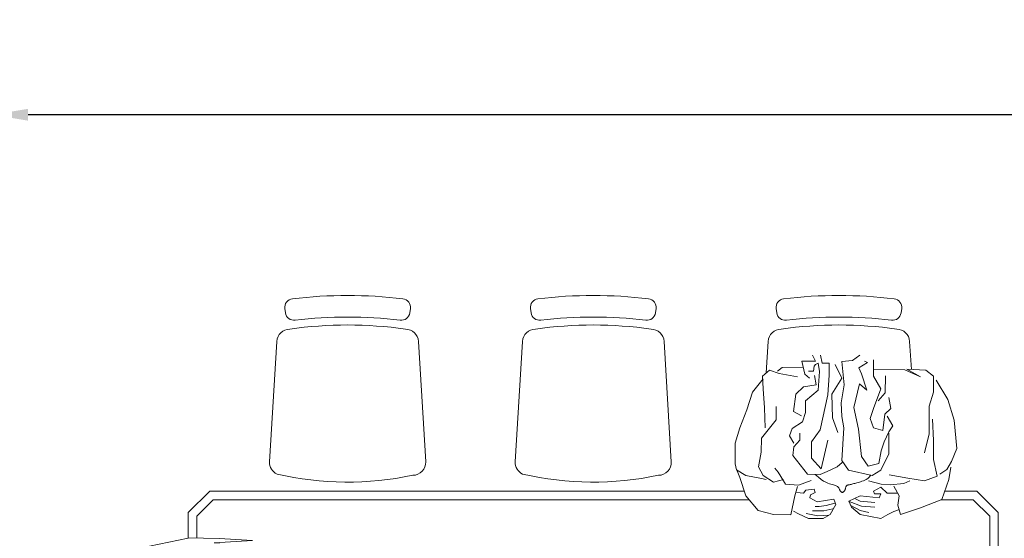
# Model space of a CAD drawing. Units: inches. Extents: x 1913 to 5309, y 1003 to 1733.
# Tile 18 of 23: x 4205 to 4275, y 1452 to 1489. Entities that reach past the tile are written whole.
import ezdxf

# ---------------------------------------------------------------- set-up
doc = ezdxf.new("R2010")
doc.units = ezdxf.units.IN
doc.layers.add('A-ANNO-DIMS', color=2, linetype='Continuous', lineweight=18)
doc.layers.add('A-FURN', color=8, linetype='Continuous', lineweight=18)
doc.styles.get("Standard").update_dxf_attribs({"font": 'arial.ttf'})
doc.dimstyles.new('ISO-25', dxfattribs={"dimtxt": 8, "dimasz": 2.5, "dimexe": 1.25, "dimexo": 0.625, "dimtad": 1, "dimdec": 1, "dimlunit": 3, "dimtxsty": 'Standard', "dimcen": 2.5, "dimclrd": 256, "dimclrt": 1, "dimadec": 0, "dimazin": 0, "dimtfac": 1, "dimtdec": 1, "dimtmove": 0, "dimatfit": 3, "dimfxl": 1, "dimarcsym": 0})

# ---------------------------------------------------------------- blocks, each defined once
blk = doc.blocks.new('A$C421907B3')
for p, q in [((1.2447, 2.3435), (1.2266, 2.4332)), ((1.4171, 1.0745), (1.4031, 1.0709)), ((1.4656, 1.0745), (1.4171, 1.0745)), ((1.5014, 1.0634), (1.4656, 1.0745)), ((1.3433, 1.0498), (1.3858, 1.0635)), ((1.3858, 1.0635), (1.4011, 1.0699)), ((1.4031, 1.0709), (1.3905, 1.0498)), ((1.5426, 1.0469), (1.5014, 1.0634)), ((1.3094, 1.0205), (1.3433, 1.0498)), ((1.3905, 1.0498), (1.3831, 1.0131)), ((1.5838, 1.034), (1.5426, 1.0469)), ((1.615, 1.0092), (1.5838, 1.034)), ((1.3001, 0.9856), (1.3094, 1.0205)), ((1.3751, 0.9856), (1.3904, 1.0094)), ((1.3831, 1.0131), (1.3811, 1.0021)), ((1.3904, 1.0094), (1.4104, 1.0204)), ((1.4104, 1.0204), (1.4443, 1.0139)), ((1.4443, 1.0139), (1.4768, 1.013)), ((1.4768, 1.013), (1.5193, 0.979)), ((1.5014, 1.0047), (1.5472, 1.0065)), ((1.5472, 1.0065), (1.5918, 1.0092)), ((1.5918, 1.0092), (1.621, 1.011)), ((1.621, 1.011), (1.6349, 0.9945)), ((1.2987, 0.9453), (1.3001, 0.9856)), ((1.3811, 0.9617), (1.3751, 0.9856)), ((1.6349, 0.9945), (1.627, 0.9725)), ((1.3705, 0.9571), (1.3877, 0.9681)), ((1.3877, 0.9681), (1.3984, 0.9745)), ((1.3984, 0.9745), (1.4077, 0.9819)), ((1.5193, 0.979), (1.5505, 0.979)), ((1.627, 0.9725), (1.6196, 0.9294)), ((1.6409, 0.9652), (1.6329, 0.9762)), ((1.6421, 0.9163), (1.6409, 0.9652)), ((1.3432, 0.9361), (1.2987, 0.9453)), ((1.3013, 0.9269), (1.3073, 0.9388)), ((1.3678, 0.9269), (1.3705, 0.9571)), ((1.3937, 0.9067), (1.4369, 0.9406)), ((1.4369, 0.9406), (1.4568, 0.9378)), ((1.4568, 0.9378), (1.4721, 0.924)), ((1.4655, 0.9378), (1.4827, 0.9479)), ((1.4827, 0.9479), (1.4994, 0.9423)), ((1.4994, 0.9423), (1.5146, 0.9176)), ((1.5286, 0.9203), (1.5392, 0.9386)), ((1.5392, 0.9386), (1.5791, 0.9331)), ((1.2907, 0.904), (1.3013, 0.9269)), ((1.3645, 0.9296), (1.3432, 0.9361)), ((1.3505, 0.9315), (1.3492, 0.9159)), ((1.3492, 0.9159), (1.3565, 0.9104)), ((1.3784, 0.8975), (1.3678, 0.9269)), ((1.4721, 0.924), (1.4887, 0.924)), ((1.5146, 0.9176), (1.5365, 0.9111)), ((1.5791, 0.9331), (1.5963, 0.9157)), ((1.5963, 0.9157), (1.601, 0.8863)), ((1.6256, 0.9129), (1.6561, 0.9193)), ((1.6561, 0.9193), (1.6561, 0.8881)), ((1.2906, 0.87), (1.2907, 0.904)), ((1.2965, 0.8821), (1.3022, 0.9091)), ((1.3079, 0.8681), (1.3079, 0.8945)), ((1.3385, 0.9012), (1.3292, 0.8838)), ((1.3458, 0.8994), (1.3385, 0.9012)), ((1.3505, 0.8883), (1.3458, 0.8994)), ((1.3565, 0.9104), (1.3584, 0.8911)), ((1.3923, 0.8773), (1.3937, 0.9067)), ((1.4056, 0.8745), (1.4302, 0.8974)), ((1.4302, 0.8974), (1.4687, 0.8974)), ((1.4687, 0.8974), (1.4966, 0.8772)), ((1.5365, 0.9111), (1.5638, 0.9111)), ((1.5638, 0.9111), (1.5883, 0.8817)), ((1.6163, 0.9019), (1.6256, 0.9129)), ((1.6329, 0.8927), (1.6329, 0.9037)), ((1.6442, 0.8908), (1.6329, 0.8927)), ((1.6561, 0.8881), (1.6701, 0.8945)), ((1.2999, 0.8535), (1.2906, 0.87)), ((1.2985, 0.8577), (1.2965, 0.8821)), ((1.3183, 0.8795), (1.3183, 0.8888)), ((1.3209, 0.8634), (1.3183, 0.8795)), ((1.3292, 0.8838), (1.3351, 0.8452)), ((1.3584, 0.8911), (1.3505, 0.8883)), ((1.3746, 0.864), (1.3774, 0.869)), ((1.3774, 0.869), (1.3812, 0.8747)), ((1.3812, 0.8747), (1.3861, 0.8811)), ((1.3861, 0.8811), (1.3923, 0.8883)), ((1.3996, 0.8608), (1.3923, 0.8773)), ((1.472, 0.8589), (1.4056, 0.8745)), ((1.4966, 0.8772), (1.5777, 0.8588)), ((1.5883, 0.8817), (1.6315, 0.8789)), ((1.601, 0.8863), (1.6222, 0.8899)), ((1.6315, 0.8789), (1.6515, 0.8817)), ((1.6481, 0.8881), (1.6442, 0.8908)), ((1.6515, 0.8817), (1.6481, 0.8881)), ((1.6514, 0.8725), (1.6701, 0.8761)), ((1.6514, 0.856), (1.6514, 0.8725)), ((1.3232, 0.8407), (1.2999, 0.8535)), ((1.3126, 0.8473), (1.3079, 0.8681)), ((1.3261, 0.8427), (1.3209, 0.8634)), ((1.368, 0.8438), (1.3687, 0.8462)), ((1.3687, 0.8462), (1.3694, 0.849)), ((1.3694, 0.849), (1.3702, 0.852)), ((1.3702, 0.852), (1.3712, 0.8555)), ((1.3712, 0.8555), (1.3726, 0.8595)), ((1.3726, 0.8595), (1.3746, 0.864)), ((1.4102, 0.8378), (1.3996, 0.8608)), ((1.49, 0.8359), (1.5239, 0.8487)), ((1.5239, 0.8487), (1.579, 0.8496)), ((1.5777, 0.8588), (1.6235, 0.856)), ((1.579, 0.8496), (1.6162, 0.8266)), ((1.6235, 0.856), (1.6514, 0.856)), ((1.3351, 0.8452), (1.3232, 0.8407)), ((1.3512, 0.826), (1.3514, 0.8269)), ((1.3512, 0.8251), (1.3512, 0.826)), ((1.3514, 0.8243), (1.3512, 0.8251)), ((1.3514, 0.8269), (1.3518, 0.8277)), ((1.3518, 0.8234), (1.3514, 0.8243)), ((1.3518, 0.8277), (1.3524, 0.8285)), ((1.3524, 0.8226), (1.3518, 0.8234)), ((1.3524, 0.8285), (1.353, 0.8292)), ((1.353, 0.8292), (1.3538, 0.8299)), ((1.3538, 0.8299), (1.3547, 0.8305)), ((1.3547, 0.8305), (1.3557, 0.8311)), ((1.3557, 0.8311), (1.3568, 0.8316)), ((1.3568, 0.8316), (1.3579, 0.832)), ((1.3579, 0.832), (1.3591, 0.8325)), ((1.3591, 0.8325), (1.3602, 0.833)), ((1.3602, 0.833), (1.3613, 0.8335)), ((1.3613, 0.8335), (1.3624, 0.8342)), ((1.3624, 0.8342), (1.3634, 0.835)), ((1.3634, 0.835), (1.3643, 0.8359)), ((1.3643, 0.8359), (1.3651, 0.837)), ((1.3651, 0.837), (1.3659, 0.8384)), ((1.3659, 0.8384), (1.3666, 0.8399)), ((1.3666, 0.8399), (1.3673, 0.8417)), ((1.3673, 0.8417), (1.368, 0.8438)), ((1.4029, 0.8112), (1.4255, 0.8268)), ((1.4208, 0.8259), (1.4102, 0.8378)), ((1.4255, 0.8268), (1.5012, 0.8222)), ((1.5012, 0.8222), (1.5272, 0.8267)), ((1.5272, 0.8267), (1.5591, 0.8285)), ((1.5591, 0.8285), (1.6009, 0.8212)), ((1.6009, 0.8212), (1.6547, 0.8266)), ((1.6162, 0.8266), (1.6481, 0.8422)), ((1.6547, 0.8266), (1.6574, 0.8018)), ((1.2999, 0.7838), (1.3165, 0.804)), ((1.3089, 0.784), (1.3203, 0.8058)), ((1.3165, 0.804), (1.3305, 0.8104)), ((1.3193, 0.7809), (1.3297, 0.8099)), ((1.3305, 0.8104), (1.3431, 0.7838)), ((1.3531, 0.8218), (1.3524, 0.8226)), ((1.354, 0.8211), (1.3531, 0.8218)), ((1.355, 0.8204), (1.354, 0.8211)), ((1.3561, 0.8198), (1.355, 0.8204)), ((1.3572, 0.8192), (1.3561, 0.8198)), ((1.3584, 0.8188), (1.3572, 0.8192)), ((1.3595, 0.8184), (1.3584, 0.8188)), ((1.3607, 0.8181), (1.3595, 0.8184)), ((1.3618, 0.8179), (1.3607, 0.8181)), ((1.3629, 0.8176), (1.3618, 0.8179)), ((1.3639, 0.8173), (1.3629, 0.8176)), ((1.3648, 0.8169), (1.3639, 0.8173)), ((1.3656, 0.8165), (1.3648, 0.8169)), ((1.3664, 0.8159), (1.3656, 0.8165)), ((1.367, 0.8151), (1.3664, 0.8159)), ((1.3675, 0.8141), (1.367, 0.8151)), ((1.3679, 0.813), (1.3675, 0.8141)), ((1.3683, 0.8118), (1.3679, 0.813)), ((1.3686, 0.8104), (1.3683, 0.8118)), ((1.369, 0.8088), (1.3686, 0.8104)), ((1.3694, 0.8071), (1.369, 0.8088)), ((1.3698, 0.8053), (1.3694, 0.8071)), ((1.3703, 0.8033), (1.3698, 0.8053)), ((1.3708, 0.8013), (1.3703, 0.8033)), ((1.3714, 0.799), (1.3708, 0.8013)), ((1.3902, 0.7562), (1.4029, 0.8112)), ((1.6574, 0.8018), (1.67, 0.7853)), ((1.2905, 0.7361), (1.2999, 0.7838)), ((1.3047, 0.7638), (1.3089, 0.784)), ((1.3166, 0.7498), (1.3193, 0.7809)), ((1.3275, 0.7498), (1.3307, 0.784)), ((1.3307, 0.784), (1.3359, 0.7949)), ((1.3431, 0.7838), (1.3384, 0.7397)), ((1.3721, 0.7967), (1.3714, 0.799)), ((1.3728, 0.7942), (1.3721, 0.7967)), ((1.3736, 0.7916), (1.3728, 0.7942)), ((1.3743, 0.7889), (1.3736, 0.7916)), ((1.3751, 0.786), (1.3743, 0.7889)), ((1.376, 0.783), (1.3751, 0.786)), ((1.3769, 0.7799), (1.376, 0.783)), ((1.378, 0.7767), (1.3769, 0.7799)), ((1.4122, 0.7654), (1.4348, 0.7809)), ((1.4348, 0.7809), (1.4979, 0.7882)), ((1.4979, 0.7882), (1.5484, 0.7992)), ((1.5484, 0.7992), (1.6035, 0.7854)), ((1.6035, 0.7854), (1.5882, 0.7689)), ((1.5882, 0.7689), (1.6268, 0.7808)), ((1.6268, 0.7808), (1.6407, 0.7872)), ((1.6407, 0.7872), (1.6527, 0.767)), ((1.3703, 0.7351), (1.3783, 0.7645)), ((1.3795, 0.7735), (1.378, 0.7767)), ((1.3813, 0.7701), (1.3795, 0.7735)), ((1.3837, 0.7667), (1.3813, 0.7701)), ((1.3866, 0.7633), (1.3837, 0.7667)), ((1.3902, 0.7599), (1.3866, 0.7633)), ((1.4028, 0.736), (1.3902, 0.7562)), ((1.4181, 0.7406), (1.4122, 0.7654)), ((1.5012, 0.7534), (1.5224, 0.7607)), ((1.5224, 0.7607), (1.5457, 0.7533)), ((1.6527, 0.767), (1.656, 0.7743)), ((1.2998, 0.7196), (1.2905, 0.7361)), ((1.3384, 0.7397), (1.3477, 0.7361)), ((1.3477, 0.7507), (1.3537, 0.7535)), ((1.3477, 0.7361), (1.3477, 0.7507)), ((1.363, 0.736), (1.349, 0.7214)), ((1.3537, 0.7535), (1.363, 0.736)), ((1.3689, 0.7149), (1.3703, 0.7351)), ((1.4407, 0.7176), (1.4028, 0.736)), ((1.4473, 0.7351), (1.4181, 0.7406)), ((1.4686, 0.7286), (1.4473, 0.7351)), ((1.4945, 0.7313), (1.5012, 0.7534)), ((1.5331, 0.7267), (1.4945, 0.7313)), ((1.5457, 0.7533), (1.5915, 0.7358)), ((1.5822, 0.7258), (1.5636, 0.7423)), ((1.5915, 0.7358), (1.6208, 0.7532)), ((1.6208, 0.7532), (1.6593, 0.7532)), ((1.6361, 0.7532), (1.636, 0.6808)), ((1.3071, 0.7058), (1.2998, 0.7196)), ((1.349, 0.7214), (1.349, 0.6984)), ((1.3716, 0.6828), (1.3689, 0.7149)), ((1.3842, 0.6736), (1.3922, 0.7167)), ((1.4885, 0.7176), (1.4407, 0.7176)), ((1.4918, 0.7176), (1.4686, 0.7286)), ((1.5058, 0.7084), (1.4918, 0.7176)), ((1.5284, 0.7212), (1.5058, 0.7084)), ((1.5457, 0.7129), (1.5331, 0.7267)), ((1.5716, 0.7175), (1.5457, 0.7129)), ((1.6221, 0.7257), (1.5822, 0.7258)), ((1.2998, 0.6902), (1.3211, 0.6966)), ((1.315, 0.6443), (1.2998, 0.6902)), ((1.3104, 0.6948), (1.3071, 0.7058)), ((1.3211, 0.6966), (1.343, 0.6939)), ((1.343, 0.6939), (1.3656, 0.7058)), ((1.3782, 0.6691), (1.3716, 0.6828)), ((1.3782, 0.6351), (1.3842, 0.6736)), ((1.636, 0.6808), (1.6194, 0.6441)), ((1.6194, 0.6441), (1.6373, 0.6762)), ((1.6373, 0.6762), (1.6346, 0.6321)), ((1.3349, 0.5948), (1.315, 0.6443)), ((1.3888, 0.6057), (1.3782, 0.6351)), ((1.4871, 0.624), (1.4426, 0.6351)), ((1.5516, 0.624), (1.4871, 0.624)), ((1.5835, 0.6138), (1.5516, 0.624)), ((1.6346, 0.6321), (1.6207, 0.6138)), ((1.3808, 0.5782), (1.3349, 0.5948)), ((1.4273, 0.614), (1.3888, 0.6057)), ((1.404, 0.5828), (1.3934, 0.5993)), ((1.4718, 0.6139), (1.4273, 0.614)), ((1.521, 0.6166), (1.4718, 0.6139)), ((1.6114, 0.6074), (1.5668, 0.5808)), ((1.6207, 0.6138), (1.5835, 0.6138)), ((1.41, 0.5736), (1.3808, 0.5782)), ((1.4226, 0.5718), (1.404, 0.5828)), ((1.4532, 0.5598), (1.4226, 0.5718)), ((1.5668, 0.5808), (1.519, 0.5662)), ((1.519, 0.5662), (1.4532, 0.5598))]:
    blk.add_line(p, q)
blk.add_lwpolyline([(1.2332, 2.2712), (1.2341, 2.2831), (1.2396, 2.1946), (1.2396, 2.1946), (1.2419, 2.2332), (1.2437, 2.2711), (1.2448, 2.3081), (1.2452, 2.3436)])
at = {"ltscale": 0.1}
for points in [[(1.2446, 2.3436), (1.3042, 2.3436), (1.3542, 2.2936), (1.3542, 1.0533)], [(1.245, 2.3234), (1.2959, 2.3236), (1.3342, 2.2853), (1.3342, 1.0419)], [(1.3342, 0.5966), (1.3342, 0.5218), (1.2959, 0.4835), (0.5125, 0.4835), (0.4742, 0.5218), (0.4742, 0.5375)], [(1.3542, 0.5878), (1.3542, 0.5135), (1.3042, 0.4635), (0.5042, 0.4635), (0.4542, 0.5135), (0.4542, 0.5377)]]:
    blk.add_lwpolyline(points, dxfattribs=at)
for points in [[(1.7302, 2.1079, 0.399285), (1.7017, 2.1378), (1.4223, 2.1548, 0.305593), (1.3936, 2.1375, 0.109362), (1.3908, 1.8225, 0.429301), (1.4223, 1.7925), (1.7017, 1.8094, 0.399285), (1.7302, 1.8394, 0.071734)], [(1.7584, 1.9736, -0.030867), (1.7509, 1.8517, 0.408428), (1.7679, 1.8294), (1.7778, 1.828, 0.419966), (1.8005, 1.8453, 0.030916), (1.8084, 1.9736, 0.030916), (1.8005, 2.1019, 0.419966), (1.7778, 2.1193), (1.7679, 2.1178, 0.408428), (1.7509, 2.0956, -0.030867)], [(1.7302, 1.5378, 0.399285), (1.7017, 1.5678), (1.4223, 1.5847, 0.305593), (1.3936, 1.5674, 0.109362), (1.3908, 1.2524, 0.429301), (1.4223, 1.2224), (1.7017, 1.2393, 0.399285), (1.7302, 1.2693, 0.071734)], [(1.7584, 1.4036, -0.030867), (1.7509, 1.2816, 0.408428), (1.7679, 1.2593), (1.7778, 1.2579, 0.419966), (1.8005, 1.2752, 0.030916), (1.8084, 1.4036, 0.030916), (1.8005, 1.5319, 0.419966), (1.7778, 1.5492), (1.7679, 1.5478, 0.408428), (1.7509, 1.5255, -0.030867)], [(1.7584, 0.8335, 0.030867), (1.7509, 0.9554, -0.408428), (1.7679, 0.9777), (1.7778, 0.9791, -0.419966), (1.8005, 0.9618, -0.030916), (1.8084, 0.8335, -0.030916), (1.8005, 0.7052, -0.419966), (1.7778, 0.6878), (1.7679, 0.6893, -0.408428), (1.7509, 0.7115, 0.030867)]]:
    blk.add_lwpolyline(points, format="xyb", close=True, dxfattribs=at)
blk.add_lwpolyline([(1.6285, 1.0021), (1.7017, 0.9977, -0.399285), (1.7302, 0.9677, -0.071734), (1.7302, 0.6992, -0.399285), (1.7017, 0.6693), (1.6367, 0.6653)], format="xyb", dxfattribs=at)
blk = doc.blocks.new('*D83')
at = {"layer": 'A-ANNO-DIMS', "color": 0, "lineweight": -2, "transparency": 16777216}
for p, q in [((4203.554, 1470.026), (4203.554, 1483.351)), ((4288.218, 1470.026), (4288.218, 1483.351))]:
    blk.add_line(p, q, dxfattribs=at)
at = {"layer": 'A-ANNO-DIMS', "lineweight": -2, "transparency": 16777216}
for p, q in [((4203.554, 1482.101), (4065.736, 1482.101)), ((4285.718, 1482.101), (4206.054, 1482.101))]:
    blk.add_line(p, q, dxfattribs=at)
at = {"layer": 'A-ANNO-DIMS', "transparency": 16777216}
for points in [[(4206.054, 1482.518), (4206.054, 1481.684), (4203.554, 1482.101)], [(4285.718, 1482.518), (4285.718, 1481.684), (4288.218, 1482.101)]]:
    blk.add_solid(points, dxfattribs=at)
at = {"layer": 'Defpoints', "color": 0, "transparency": 16777216}
for p in [(4203.554, 1482.101), (4203.554, 1469.401), (4288.218, 1469.401)]:
    blk.add_point(p, dxfattribs=at)
at = {"layer": 'A-ANNO-DIMS', "color": 1, "transparency": 16777216, "insert": (4133.395, 1486.862), "char_height": 8, "attachment_point": 5}
blk.add_mtext('DINING SET 7\'-0 1/2" TYP.', dxfattribs=at)

msp = doc.modelspace()

# ---------------------------------------------------------------- block references
at = {"layer": 'A-FURN', "xscale": 30.26057373645948, "yscale": 30.26057373645948, "zscale": 30.26057373645948, "rotation": 89.99999999999996}
msp.add_blockref('A$C421907B3', (4288.218, 1414.678), dxfattribs=at)

# ---------------------------------------------------------------- dimensions: what is measured, and where the dimension line sits
at = {"layer": 'A-ANNO-DIMS'}
dim = msp.add_linear_dim(base=(4203.554, 1482.101), p1=(4288.218, 1469.401), p2=(4203.554, 1469.401), angle=180, text='DINING SET <> TYP.', dimstyle='ISO-25', override={"dimdec": 1, "dimrnd": 0, "dimzin": 1, "dimlunit": 4, "dimfrac": 2}, dxfattribs=at)
dim.commit()
dim.dimension.update_dxf_attribs({"geometry": '*D83', "text_midpoint": (4133.395, 1486.862)})

doc.saveas('drawing.dxf')
